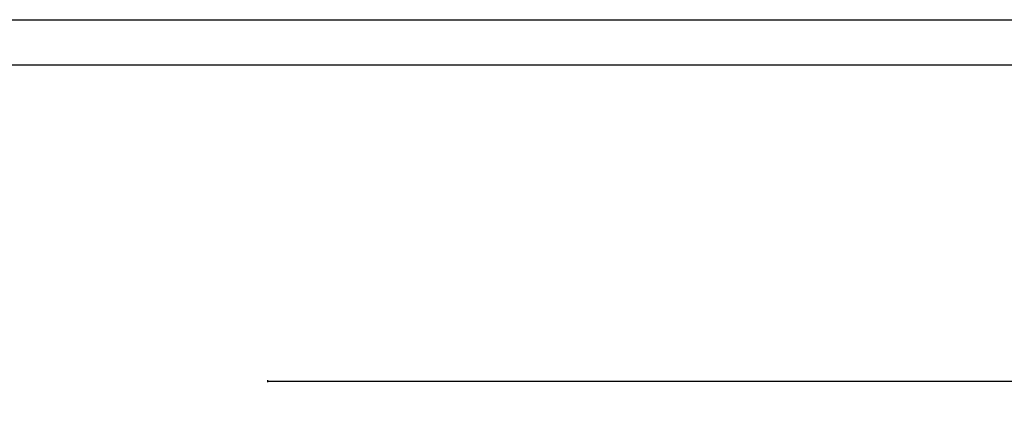
# Model space of a CAD drawing. Units: inches. Extents: x 0 to 4258, y 0 to 3769.
# Tile 24 of 30: x 3623 to 3845, y 3682 to 3769. Entities that reach past the tile are written whole.
import ezdxf

# ---------------------------------------------------------------- set-up
doc = ezdxf.new("R2010")
doc.units = ezdxf.units.IN
doc.header["$MEASUREMENT"] = 0
doc.layers.add('A-ANNO-DIMS', color=250, linetype='Continuous', lineweight=18)
doc.layers.add('A-ANNO-TTLB', color=250, linetype='Continuous', lineweight=25)
doc.styles.get("Standard").update_dxf_attribs({"font": 'arial.ttf'})
doc.dimstyles.get("Standard").update_dxf_attribs({"dimtxt": 7, "dimasz": 0.18, "dimexe": 0.18, "dimexo": 0.0625, "dimgap": 0.09, "dimtad": 0, "dimtih": 1, "dimtoh": 1, "dimzin": 0, "dimdsep": 46, "dimlunit": 3, "dimtxsty": 'Standard', "dimcen": 0.09, "dimadec": 0, "dimazin": 0, "dimtfac": 1, "dimtofl": 0, "dimtmove": 0, "dimatfit": 3, "dimfxl": 1, "dimtolj": 1, "dimtzin": 0, "dimarcsym": 0})

# ---------------------------------------------------------------- blocks, each defined once
blk = doc.blocks.new('*D24')
at = {"layer": 'A-ANNO-DIMS', "color": 0, "lineweight": -2, "transparency": 16777216}
for p, q in [((3678.8, 3686.57), (3678.8, 3687.02)), ((4038.8, 3686.57), (4038.8, 3687.02)), ((3678.98, 3686.84), (3852.78, 3686.84)), ((4038.62, 3686.84), (3864.83, 3686.84))]:
    blk.add_line(p, q, dxfattribs=at)
at = {"layer": 'A-ANNO-DIMS', "color": 0, "transparency": 16777216}
for points in [[(3678.98, 3686.87), (3678.98, 3686.81), (3678.8, 3686.84)], [(4038.62, 3686.87), (4038.62, 3686.81), (4038.8, 3686.84)]]:
    blk.add_solid(points, dxfattribs=at)
at = {"layer": 'Defpoints', "color": 0, "transparency": 16777216}
for p in [(3678.8, 3686.51), (4038.8, 3686.84), (4038.8, 3686.51)]:
    blk.add_point(p, dxfattribs=at)
at = {"layer": 'A-ANNO-DIMS', "color": 0, "transparency": 16777216, "insert": (3858.8, 3686.84), "char_height": 7, "attachment_point": 5}
blk.add_mtext("\\A1;30'", dxfattribs=at)

msp = doc.modelspace()

# ---------------------------------------------------------------- linework, layer by layer
at = {"layer": 'A-ANNO-TTLB'}
for p, q in [((3476.156, 3768.679), (4257.673, 3768.679)), ((4244.279, 3758.41), (3489.722, 3758.41))]:
    msp.add_line(p, q, dxfattribs=at)

# ---------------------------------------------------------------- dimensions: what is measured, and where the dimension line sits
at = {"layer": 'A-ANNO-DIMS'}
dim = msp.add_linear_dim(base=(4038.804, 3686.844), p1=(3678.804, 3686.506), p2=(4038.804, 3686.506), dimstyle='Standard', override={"dimclrd": 0, "dimclre": 0, "dimclrt": 0}, dxfattribs=at)
dim.commit()
dim.dimension.update_dxf_attribs({"geometry": '*D24', "text_midpoint": (3858.804, 3686.844)})

doc.saveas('drawing.dxf')
